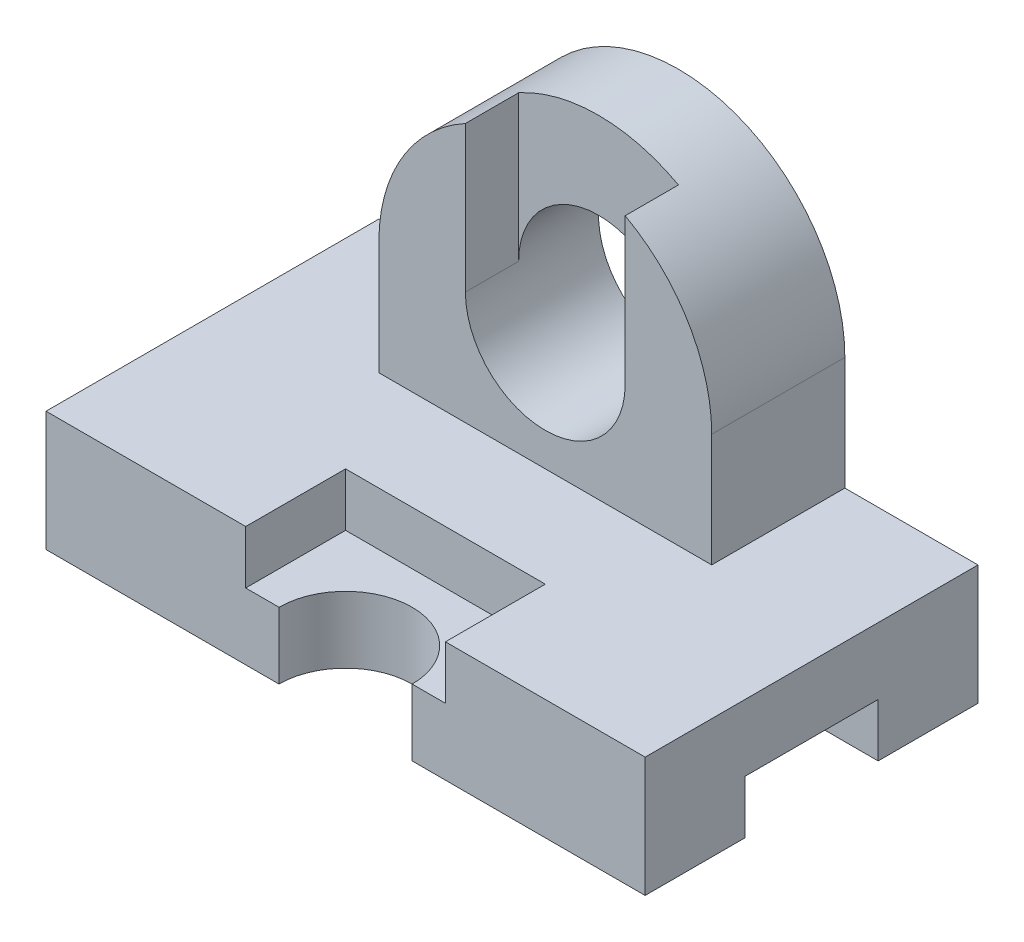
ISO-10303-21;
HEADER;
FILE_DESCRIPTION(('STEP AP214'),'2;1');
FILE_NAME('part.step','',(''),(''),'','','');
FILE_SCHEMA(('AUTOMOTIVE_DESIGN { 1 0 10303 214 1 1 1 1 }'));
ENDSEC;
DATA;
#1=APPLICATION_CONTEXT('core data for automotive mechanical design processes');
#2=APPLICATION_PROTOCOL_DEFINITION('international standard','automotive_design',2000,#1);
#3=PRODUCT_CONTEXT('',#1,'mechanical');
#4=PRODUCT('Part','Part','',(#3));
#5=PRODUCT_RELATED_PRODUCT_CATEGORY('part','',(#4));
#6=PRODUCT_DEFINITION_FORMATION('','',#4);
#7=PRODUCT_DEFINITION_CONTEXT('part definition',#1,'design');
#8=PRODUCT_DEFINITION('design','',#6,#7);
#9=PRODUCT_DEFINITION_SHAPE('','',#8);
#10=(LENGTH_UNIT() NAMED_UNIT(*) SI_UNIT(.MILLI.,.METRE.));
#11=(NAMED_UNIT(*) PLANE_ANGLE_UNIT() SI_UNIT($,.RADIAN.));
#12=(NAMED_UNIT(*) SI_UNIT($,.STERADIAN.) SOLID_ANGLE_UNIT());
#13=UNCERTAINTY_MEASURE_WITH_UNIT(LENGTH_MEASURE(1.E-05),#10,'distance_accuracy_value','');
#14=(GEOMETRIC_REPRESENTATION_CONTEXT(3) GLOBAL_UNCERTAINTY_ASSIGNED_CONTEXT((#13)) GLOBAL_UNIT_ASSIGNED_CONTEXT((#10,
#11,#12)) REPRESENTATION_CONTEXT('',''));
#15=CARTESIAN_POINT('',(0.,0.,0.));
#16=DIRECTION('',(0.,0.,1.));
#17=DIRECTION('',(1.,0.,0.));
#18=AXIS2_PLACEMENT_3D('',#15,#16,#17);
#19=CARTESIAN_POINT('',(0.,0.,50.));
#20=DIRECTION('',(0.,0.,1.));
#21=DIRECTION('',(1.,0.,0.));
#22=AXIS2_PLACEMENT_3D('',#19,#20,#21);
#23=PLANE('',#22);
#24=DIRECTION('',(0.,1.,0.));
#25=VECTOR('',#24,1.);
#26=CARTESIAN_POINT('',(55.,0.,50.));
#27=LINE('',#26,#25);
#28=CARTESIAN_POINT('',(55.,0.,50.));
#29=VERTEX_POINT('',#28);
#30=CARTESIAN_POINT('',(55.,10.,50.));
#31=VERTEX_POINT('',#30);
#32=EDGE_CURVE('E57',#29,#31,#27,.T.);
#33=ORIENTED_EDGE('',*,*,#32,.F.);
#34=DIRECTION('',(1.,0.,0.));
#35=VECTOR('',#34,1.);
#36=CARTESIAN_POINT('',(0.,0.,50.));
#37=LINE('',#36,#35);
#38=CARTESIAN_POINT('',(90.,0.,50.));
#39=VERTEX_POINT('',#38);
#40=EDGE_CURVE('E201',#29,#39,#37,.T.);
#41=ORIENTED_EDGE('',*,*,#40,.T.);
#42=DIRECTION('',(0.,1.,0.));
#43=VECTOR('',#42,1.);
#44=CARTESIAN_POINT('',(90.,0.,50.));
#45=LINE('',#44,#43);
#46=CARTESIAN_POINT('',(90.,18.,50.));
#47=VERTEX_POINT('',#46);
#48=EDGE_CURVE('E213',#39,#47,#45,.T.);
#49=ORIENTED_EDGE('',*,*,#48,.T.);
#50=DIRECTION('',(-1.,0.,0.));
#51=VECTOR('',#50,1.);
#52=CARTESIAN_POINT('',(90.,18.,50.));
#53=LINE('',#52,#51);
#54=CARTESIAN_POINT('',(60.,18.,50.));
#55=VERTEX_POINT('',#54);
#56=EDGE_CURVE('E223',#47,#55,#53,.T.);
#57=ORIENTED_EDGE('',*,*,#56,.T.);
#58=DIRECTION('',(0.,1.,0.));
#59=VECTOR('',#58,1.);
#60=CARTESIAN_POINT('',(60.,10.,50.));
#61=LINE('',#60,#59);
#62=CARTESIAN_POINT('',(60.,10.,50.));
#63=VERTEX_POINT('',#62);
#64=EDGE_CURVE('E273',#63,#55,#61,.T.);
#65=ORIENTED_EDGE('',*,*,#64,.F.);
#66=DIRECTION('',(1.,0.,0.));
#67=VECTOR('',#66,1.);
#68=CARTESIAN_POINT('',(30.,10.,50.));
#69=LINE('',#68,#67);
#70=EDGE_CURVE('E202',#31,#63,#69,.T.);
#71=ORIENTED_EDGE('',*,*,#70,.F.);
#72=EDGE_LOOP('',(#33,#41,#49,#57,#65,#71));
#73=FACE_BOUND('',#72,.T.);
#74=ADVANCED_FACE('F41',(#73),#23,.T.);
#75=CARTESIAN_POINT('',(0.,0.,50.));
#76=DIRECTION('',(0.,1.,0.));
#77=DIRECTION('',(0.,0.,1.));
#78=AXIS2_PLACEMENT_3D('',#75,#76,#77);
#79=PLANE('',#78);
#80=ORIENTED_EDGE('',*,*,#40,.F.);
#81=CARTESIAN_POINT('',(45.,0.,50.));
#82=DIRECTION('',(0.,1.,0.));
#83=DIRECTION('',(0.,0.,1.));
#84=AXIS2_PLACEMENT_3D('',#81,#82,#83);
#85=CIRCLE('',#84,10.);
#86=CARTESIAN_POINT('',(35.,0.,50.));
#87=VERTEX_POINT('',#86);
#88=EDGE_CURVE('E188',#29,#87,#85,.T.);
#89=ORIENTED_EDGE('',*,*,#88,.T.);
#90=CARTESIAN_POINT('',(0.,0.,50.));
#91=VERTEX_POINT('',#90);
#92=EDGE_CURVE('E215',#91,#87,#37,.T.);
#93=ORIENTED_EDGE('',*,*,#92,.F.);
#94=DIRECTION('',(0.,0.,-1.));
#95=VECTOR('',#94,1.);
#96=CARTESIAN_POINT('',(0.,0.,50.));
#97=LINE('',#96,#95);
#98=CARTESIAN_POINT('',(0.,0.,35.));
#99=VERTEX_POINT('',#98);
#100=EDGE_CURVE('E11',#91,#99,#97,.T.);
#101=ORIENTED_EDGE('',*,*,#100,.T.);
#102=DIRECTION('',(1.,0.,0.));
#103=VECTOR('',#102,1.);
#104=CARTESIAN_POINT('',(0.,0.,35.));
#105=LINE('',#104,#103);
#106=CARTESIAN_POINT('',(90.,0.,35.));
#107=VERTEX_POINT('',#106);
#108=EDGE_CURVE('E335',#99,#107,#105,.T.);
#109=ORIENTED_EDGE('',*,*,#108,.T.);
#110=DIRECTION('',(0.,0.,-1.));
#111=VECTOR('',#110,1.);
#112=CARTESIAN_POINT('',(90.,0.,50.));
#113=LINE('',#112,#111);
#114=EDGE_CURVE('E208',#39,#107,#113,.T.);
#115=ORIENTED_EDGE('',*,*,#114,.F.);
#116=EDGE_LOOP('',(#80,#89,#93,#101,#109,#115));
#117=FACE_BOUND('',#116,.T.);
#118=ADVANCED_FACE('F210',(#117),#79,.F.);
#119=CARTESIAN_POINT('',(90.,18.,50.));
#120=DIRECTION('',(0.,-1.,0.));
#121=DIRECTION('',(0.,0.,-1.));
#122=AXIS2_PLACEMENT_3D('',#119,#120,#121);
#123=PLANE('',#122);
#124=DIRECTION('',(-1.,0.,0.));
#125=VECTOR('',#124,1.);
#126=CARTESIAN_POINT('',(30.,18.,35.));
#127=LINE('',#126,#125);
#128=CARTESIAN_POINT('',(60.,18.,35.));
#129=VERTEX_POINT('',#128);
#130=CARTESIAN_POINT('',(30.,18.,35.));
#131=VERTEX_POINT('',#130);
#132=EDGE_CURVE('E386',#129,#131,#127,.T.);
#133=ORIENTED_EDGE('',*,*,#132,.F.);
#134=DIRECTION('',(0.,0.,-1.));
#135=VECTOR('',#134,1.);
#136=CARTESIAN_POINT('',(60.,18.,35.));
#137=LINE('',#136,#135);
#138=EDGE_CURVE('E204',#55,#129,#137,.T.);
#139=ORIENTED_EDGE('',*,*,#138,.F.);
#140=ORIENTED_EDGE('',*,*,#56,.F.);
#141=DIRECTION('',(0.,0.,-1.));
#142=VECTOR('',#141,1.);
#143=CARTESIAN_POINT('',(90.,18.,50.));
#144=LINE('',#143,#142);
#145=CARTESIAN_POINT('',(90.,18.,0.));
#146=VERTEX_POINT('',#145);
#147=EDGE_CURVE('E241',#47,#146,#144,.T.);
#148=ORIENTED_EDGE('',*,*,#147,.T.);
#149=DIRECTION('',(-1.,0.,0.));
#150=VECTOR('',#149,1.);
#151=CARTESIAN_POINT('',(90.,18.,0.));
#152=LINE('',#151,#150);
#153=CARTESIAN_POINT('',(70.,18.,0.));
#154=VERTEX_POINT('',#153);
#155=EDGE_CURVE('E220',#146,#154,#152,.T.);
#156=ORIENTED_EDGE('',*,*,#155,.T.);
#157=DIRECTION('',(0.,0.,-1.));
#158=VECTOR('',#157,1.);
#159=CARTESIAN_POINT('',(70.,18.,20.));
#160=LINE('',#159,#158);
#161=CARTESIAN_POINT('',(70.,18.,20.));
#162=VERTEX_POINT('',#161);
#163=EDGE_CURVE('E275',#162,#154,#160,.T.);
#164=ORIENTED_EDGE('',*,*,#163,.F.);
#165=DIRECTION('',(1.,0.,0.));
#166=VECTOR('',#165,1.);
#167=CARTESIAN_POINT('',(20.,18.,20.));
#168=LINE('',#167,#166);
#169=CARTESIAN_POINT('',(20.,18.,20.));
#170=VERTEX_POINT('',#169);
#171=EDGE_CURVE('E355',#170,#162,#168,.T.);
#172=ORIENTED_EDGE('',*,*,#171,.F.);
#173=DIRECTION('',(0.,0.,-1.));
#174=VECTOR('',#173,1.);
#175=CARTESIAN_POINT('',(20.,18.,20.));
#176=LINE('',#175,#174);
#177=CARTESIAN_POINT('',(20.,18.,0.));
#178=VERTEX_POINT('',#177);
#179=EDGE_CURVE('E362',#170,#178,#176,.T.);
#180=ORIENTED_EDGE('',*,*,#179,.T.);
#181=CARTESIAN_POINT('',(0.,18.,0.));
#182=VERTEX_POINT('',#181);
#183=EDGE_CURVE('E236',#178,#182,#152,.T.);
#184=ORIENTED_EDGE('',*,*,#183,.T.);
#185=DIRECTION('',(0.,0.,-1.));
#186=VECTOR('',#185,1.);
#187=CARTESIAN_POINT('',(0.,18.,50.));
#188=LINE('',#187,#186);
#189=CARTESIAN_POINT('',(0.,18.,50.));
#190=VERTEX_POINT('',#189);
#191=EDGE_CURVE('E228',#190,#182,#188,.T.);
#192=ORIENTED_EDGE('',*,*,#191,.F.);
#193=CARTESIAN_POINT('',(30.,18.,50.));
#194=VERTEX_POINT('',#193);
#195=EDGE_CURVE('E225',#194,#190,#53,.T.);
#196=ORIENTED_EDGE('',*,*,#195,.F.);
#197=DIRECTION('',(0.,0.,1.));
#198=VECTOR('',#197,1.);
#199=CARTESIAN_POINT('',(30.,18.,35.));
#200=LINE('',#199,#198);
#201=EDGE_CURVE('E288',#131,#194,#200,.T.);
#202=ORIENTED_EDGE('',*,*,#201,.F.);
#203=EDGE_LOOP('',(#133,#139,#140,#148,#156,#164,#172,#180,#184,#192,#196,#202));
#204=FACE_BOUND('',#203,.T.);
#205=ADVANCED_FACE('F269',(#204),#123,.F.);
#206=CARTESIAN_POINT('',(0.,18.,50.));
#207=DIRECTION('',(1.,0.,0.));
#208=DIRECTION('',(0.,0.,-1.));
#209=AXIS2_PLACEMENT_3D('',#206,#207,#208);
#210=PLANE('',#209);
#211=DIRECTION('',(0.,0.,1.));
#212=VECTOR('',#211,1.);
#213=CARTESIAN_POINT('',(0.,8.,35.));
#214=LINE('',#213,#212);
#215=CARTESIAN_POINT('',(0.,8.,15.));
#216=VERTEX_POINT('',#215);
#217=CARTESIAN_POINT('',(0.,8.,35.));
#218=VERTEX_POINT('',#217);
#219=EDGE_CURVE('E316',#216,#218,#214,.T.);
#220=ORIENTED_EDGE('',*,*,#219,.T.);
#221=DIRECTION('',(0.,-1.,0.));
#222=VECTOR('',#221,1.);
#223=CARTESIAN_POINT('',(0.,0.,35.));
#224=LINE('',#223,#222);
#225=EDGE_CURVE('E324',#218,#99,#224,.T.);
#226=ORIENTED_EDGE('',*,*,#225,.T.);
#227=ORIENTED_EDGE('',*,*,#100,.F.);
#228=DIRECTION('',(0.,-1.,0.));
#229=VECTOR('',#228,1.);
#230=CARTESIAN_POINT('',(0.,18.,50.));
#231=LINE('',#230,#229);
#232=EDGE_CURVE('E214',#190,#91,#231,.T.);
#233=ORIENTED_EDGE('',*,*,#232,.F.);
#234=ORIENTED_EDGE('',*,*,#191,.T.);
#235=DIRECTION('',(0.,-1.,0.));
#236=VECTOR('',#235,1.);
#237=CARTESIAN_POINT('',(0.,18.,0.));
#238=LINE('',#237,#236);
#239=CARTESIAN_POINT('',(0.,0.,0.));
#240=VERTEX_POINT('',#239);
#241=EDGE_CURVE('E227',#182,#240,#238,.T.);
#242=ORIENTED_EDGE('',*,*,#241,.T.);
#243=CARTESIAN_POINT('',(0.,0.,15.));
#244=VERTEX_POINT('',#243);
#245=EDGE_CURVE('E47',#244,#240,#97,.T.);
#246=ORIENTED_EDGE('',*,*,#245,.F.);
#247=DIRECTION('',(0.,1.,0.));
#248=VECTOR('',#247,1.);
#249=CARTESIAN_POINT('',(0.,8.,15.));
#250=LINE('',#249,#248);
#251=EDGE_CURVE('E317',#244,#216,#250,.T.);
#252=ORIENTED_EDGE('',*,*,#251,.T.);
#253=EDGE_LOOP('',(#220,#226,#227,#233,#234,#242,#246,#252));
#254=FACE_BOUND('',#253,.T.);
#255=ADVANCED_FACE('F43',(#254),#210,.F.);
#256=CARTESIAN_POINT('',(90.,0.,15.));
#257=VERTEX_POINT('',#256);
#258=CARTESIAN_POINT('',(90.,0.,0.));
#259=VERTEX_POINT('',#258);
#260=EDGE_CURVE('E243',#257,#259,#113,.T.);
#261=ORIENTED_EDGE('',*,*,#260,.F.);
#262=DIRECTION('',(1.,0.,0.));
#263=VECTOR('',#262,1.);
#264=CARTESIAN_POINT('',(0.,0.,15.));
#265=LINE('',#264,#263);
#266=EDGE_CURVE('E326',#244,#257,#265,.T.);
#267=ORIENTED_EDGE('',*,*,#266,.F.);
#268=ORIENTED_EDGE('',*,*,#245,.T.);
#269=DIRECTION('',(1.,0.,0.));
#270=VECTOR('',#269,1.);
#271=CARTESIAN_POINT('',(0.,0.,0.));
#272=LINE('',#271,#270);
#273=EDGE_CURVE('E229',#240,#259,#272,.T.);
#274=ORIENTED_EDGE('',*,*,#273,.T.);
#275=EDGE_LOOP('',(#261,#267,#268,#274));
#276=FACE_BOUND('',#275,.T.);
#277=ADVANCED_FACE('F260',(#276),#79,.F.);
#278=CARTESIAN_POINT('',(90.,0.,50.));
#279=DIRECTION('',(-1.,0.,0.));
#280=DIRECTION('',(0.,0.,1.));
#281=AXIS2_PLACEMENT_3D('',#278,#279,#280);
#282=PLANE('',#281);
#283=ORIENTED_EDGE('',*,*,#114,.T.);
#284=DIRECTION('',(0.,-1.,0.));
#285=VECTOR('',#284,1.);
#286=CARTESIAN_POINT('',(90.,0.,35.));
#287=LINE('',#286,#285);
#288=CARTESIAN_POINT('',(90.,8.,35.));
#289=VERTEX_POINT('',#288);
#290=EDGE_CURVE('E318',#289,#107,#287,.T.);
#291=ORIENTED_EDGE('',*,*,#290,.F.);
#292=DIRECTION('',(0.,0.,1.));
#293=VECTOR('',#292,1.);
#294=CARTESIAN_POINT('',(90.,8.,35.));
#295=LINE('',#294,#293);
#296=CARTESIAN_POINT('',(90.,8.,15.));
#297=VERTEX_POINT('',#296);
#298=EDGE_CURVE('E328',#297,#289,#295,.T.);
#299=ORIENTED_EDGE('',*,*,#298,.F.);
#300=DIRECTION('',(0.,1.,0.));
#301=VECTOR('',#300,1.);
#302=CARTESIAN_POINT('',(90.,8.,15.));
#303=LINE('',#302,#301);
#304=EDGE_CURVE('E254',#257,#297,#303,.T.);
#305=ORIENTED_EDGE('',*,*,#304,.F.);
#306=ORIENTED_EDGE('',*,*,#260,.T.);
#307=DIRECTION('',(0.,1.,0.));
#308=VECTOR('',#307,1.);
#309=CARTESIAN_POINT('',(90.,0.,0.));
#310=LINE('',#309,#308);
#311=EDGE_CURVE('E234',#259,#146,#310,.T.);
#312=ORIENTED_EDGE('',*,*,#311,.T.);
#313=ORIENTED_EDGE('',*,*,#147,.F.);
#314=ORIENTED_EDGE('',*,*,#48,.F.);
#315=EDGE_LOOP('',(#283,#291,#299,#305,#306,#312,#313,#314));
#316=FACE_BOUND('',#315,.T.);
#317=ADVANCED_FACE('F247',(#316),#282,.F.);
#318=DIRECTION('',(0.,1.,0.));
#319=VECTOR('',#318,1.);
#320=CARTESIAN_POINT('',(35.,0.,50.));
#321=LINE('',#320,#319);
#322=CARTESIAN_POINT('',(35.,10.,50.));
#323=VERTEX_POINT('',#322);
#324=EDGE_CURVE('E194',#323,#87,#321,.F.);
#325=ORIENTED_EDGE('',*,*,#324,.F.);
#326=CARTESIAN_POINT('',(30.,10.,50.));
#327=VERTEX_POINT('',#326);
#328=EDGE_CURVE('E295',#327,#323,#69,.T.);
#329=ORIENTED_EDGE('',*,*,#328,.F.);
#330=DIRECTION('',(0.,1.,0.));
#331=VECTOR('',#330,1.);
#332=CARTESIAN_POINT('',(30.,10.,50.));
#333=LINE('',#332,#331);
#334=EDGE_CURVE('E278',#327,#194,#333,.T.);
#335=ORIENTED_EDGE('',*,*,#334,.T.);
#336=ORIENTED_EDGE('',*,*,#195,.T.);
#337=ORIENTED_EDGE('',*,*,#232,.T.);
#338=ORIENTED_EDGE('',*,*,#92,.T.);
#339=EDGE_LOOP('',(#325,#329,#335,#336,#337,#338));
#340=FACE_BOUND('',#339,.T.);
#341=ADVANCED_FACE('F383',(#340),#23,.T.);
#342=CARTESIAN_POINT('',(0.,0.,0.));
#343=DIRECTION('',(0.,0.,1.));
#344=DIRECTION('',(1.,0.,0.));
#345=AXIS2_PLACEMENT_3D('',#342,#343,#344);
#346=PLANE('',#345);
#347=ORIENTED_EDGE('',*,*,#241,.F.);
#348=ORIENTED_EDGE('',*,*,#183,.F.);
#349=DIRECTION('',(0.,-1.,0.));
#350=VECTOR('',#349,1.);
#351=CARTESIAN_POINT('',(20.,35.,0.));
#352=LINE('',#351,#350);
#353=CARTESIAN_POINT('',(20.,35.,0.));
#354=VERTEX_POINT('',#353);
#355=EDGE_CURVE('E360',#354,#178,#352,.T.);
#356=ORIENTED_EDGE('',*,*,#355,.F.);
#357=CARTESIAN_POINT('',(45.,35.,0.));
#358=DIRECTION('',(0.,0.,1.));
#359=DIRECTION('',(1.,0.,0.));
#360=AXIS2_PLACEMENT_3D('',#357,#358,#359);
#361=CIRCLE('',#360,25.);
#362=CARTESIAN_POINT('',(70.,35.,0.));
#363=VERTEX_POINT('',#362);
#364=EDGE_CURVE('E344',#363,#354,#361,.T.);
#365=ORIENTED_EDGE('',*,*,#364,.F.);
#366=DIRECTION('',(0.,1.,0.));
#367=VECTOR('',#366,1.);
#368=CARTESIAN_POINT('',(70.,35.,0.));
#369=LINE('',#368,#367);
#370=EDGE_CURVE('E266',#154,#363,#369,.T.);
#371=ORIENTED_EDGE('',*,*,#370,.F.);
#372=ORIENTED_EDGE('',*,*,#155,.F.);
#373=ORIENTED_EDGE('',*,*,#311,.F.);
#374=ORIENTED_EDGE('',*,*,#273,.F.);
#375=EDGE_LOOP('',(#347,#348,#356,#365,#371,#372,#373,#374));
#376=FACE_BOUND('',#375,.T.);
#377=CARTESIAN_POINT('',(45.,35.,0.));
#378=DIRECTION('',(0.,0.,1.));
#379=DIRECTION('',(1.,0.,0.));
#380=AXIS2_PLACEMENT_3D('',#377,#378,#379);
#381=CIRCLE('',#380,12.);
#382=CARTESIAN_POINT('',(57.,35.,0.));
#383=VERTEX_POINT('',#382);
#384=EDGE_CURVE('E332',#383,#383,#381,.T.);
#385=ORIENTED_EDGE('',*,*,#384,.T.);
#386=EDGE_LOOP('',(#385));
#387=FACE_BOUND('',#386,.T.);
#388=ADVANCED_FACE('F265',(#376,#387),#346,.F.);
#389=CARTESIAN_POINT('',(45.,35.,20.));
#390=DIRECTION('',(0.,0.,1.));
#391=DIRECTION('',(1.,0.,0.));
#392=AXIS2_PLACEMENT_3D('',#389,#390,#391);
#393=PLANE('',#392);
#394=DIRECTION('',(0.,-1.,0.));
#395=VECTOR('',#394,1.);
#396=CARTESIAN_POINT('',(33.,35.,20.));
#397=LINE('',#396,#395);
#398=CARTESIAN_POINT('',(33.,56.9317121994613,20.));
#399=VERTEX_POINT('',#398);
#400=CARTESIAN_POINT('',(33.,35.,20.));
#401=VERTEX_POINT('',#400);
#402=EDGE_CURVE('E285',#399,#401,#397,.T.);
#403=ORIENTED_EDGE('',*,*,#402,.F.);
#404=CARTESIAN_POINT('',(45.,35.,20.));
#405=DIRECTION('',(0.,0.,1.));
#406=DIRECTION('',(1.,0.,0.));
#407=AXIS2_PLACEMENT_3D('',#404,#405,#406);
#408=CIRCLE('',#407,25.);
#409=CARTESIAN_POINT('',(20.,35.,20.));
#410=VERTEX_POINT('',#409);
#411=EDGE_CURVE('E349',#399,#410,#408,.T.);
#412=ORIENTED_EDGE('',*,*,#411,.T.);
#413=DIRECTION('',(0.,-1.,0.));
#414=VECTOR('',#413,1.);
#415=CARTESIAN_POINT('',(20.,35.,20.));
#416=LINE('',#415,#414);
#417=EDGE_CURVE('E347',#410,#170,#416,.T.);
#418=ORIENTED_EDGE('',*,*,#417,.T.);
#419=ORIENTED_EDGE('',*,*,#171,.T.);
#420=DIRECTION('',(0.,1.,0.));
#421=VECTOR('',#420,1.);
#422=CARTESIAN_POINT('',(70.,35.,20.));
#423=LINE('',#422,#421);
#424=CARTESIAN_POINT('',(70.,35.,20.));
#425=VERTEX_POINT('',#424);
#426=EDGE_CURVE('E352',#162,#425,#423,.T.);
#427=ORIENTED_EDGE('',*,*,#426,.T.);
#428=CARTESIAN_POINT('',(57.,56.9317121994613,20.));
#429=VERTEX_POINT('',#428);
#430=EDGE_CURVE('E346',#425,#429,#408,.T.);
#431=ORIENTED_EDGE('',*,*,#430,.T.);
#432=DIRECTION('',(0.,1.,0.));
#433=VECTOR('',#432,1.);
#434=CARTESIAN_POINT('',(57.,35.,20.));
#435=LINE('',#434,#433);
#436=CARTESIAN_POINT('',(57.,35.,20.));
#437=VERTEX_POINT('',#436);
#438=EDGE_CURVE('E276',#437,#429,#435,.T.);
#439=ORIENTED_EDGE('',*,*,#438,.F.);
#440=CARTESIAN_POINT('',(45.,35.,20.));
#441=DIRECTION('',(0.,0.,1.));
#442=DIRECTION('',(1.,0.,0.));
#443=AXIS2_PLACEMENT_3D('',#440,#441,#442);
#444=CIRCLE('',#443,12.);
#445=EDGE_CURVE('E338',#401,#437,#444,.T.);
#446=ORIENTED_EDGE('',*,*,#445,.F.);
#447=EDGE_LOOP('',(#403,#412,#418,#419,#427,#431,#439,#446));
#448=FACE_BOUND('',#447,.T.);
#449=ADVANCED_FACE('F424',(#448),#393,.T.);
#450=CARTESIAN_POINT('',(45.,35.,20.));
#451=DIRECTION('',(0.,0.,-1.));
#452=DIRECTION('',(-1.,0.,0.));
#453=AXIS2_PLACEMENT_3D('',#450,#451,#452);
#454=CYLINDRICAL_SURFACE('',#453,25.);
#455=ORIENTED_EDGE('',*,*,#411,.F.);
#456=DIRECTION('',(0.,0.,1.));
#457=VECTOR('',#456,1.);
#458=CARTESIAN_POINT('',(33.,56.9317121994613,12.));
#459=LINE('',#458,#457);
#460=CARTESIAN_POINT('',(33.,56.9317121994613,12.));
#461=VERTEX_POINT('',#460);
#462=EDGE_CURVE('E309',#461,#399,#459,.T.);
#463=ORIENTED_EDGE('',*,*,#462,.F.);
#464=CARTESIAN_POINT('',(45.,34.9999999999993,12.));
#465=DIRECTION('',(0.,0.,1.));
#466=DIRECTION('',(-1.,0.,0.));
#467=AXIS2_PLACEMENT_3D('',#464,#465,#466);
#468=CIRCLE('',#467,25.0000000000006);
#469=CARTESIAN_POINT('',(57.,56.9317121994613,12.));
#470=VERTEX_POINT('',#469);
#471=EDGE_CURVE('E301',#470,#461,#468,.T.);
#472=ORIENTED_EDGE('',*,*,#471,.F.);
#473=DIRECTION('',(0.,0.,1.));
#474=VECTOR('',#473,1.);
#475=CARTESIAN_POINT('',(57.,56.9317121994613,12.));
#476=LINE('',#475,#474);
#477=EDGE_CURVE('E315',#470,#429,#476,.T.);
#478=ORIENTED_EDGE('',*,*,#477,.T.);
#479=ORIENTED_EDGE('',*,*,#430,.F.);
#480=DIRECTION('',(0.,0.,-1.));
#481=VECTOR('',#480,1.);
#482=CARTESIAN_POINT('',(70.,35.,20.));
#483=LINE('',#482,#481);
#484=EDGE_CURVE('E358',#425,#363,#483,.T.);
#485=ORIENTED_EDGE('',*,*,#484,.T.);
#486=ORIENTED_EDGE('',*,*,#364,.T.);
#487=DIRECTION('',(0.,0.,-1.));
#488=VECTOR('',#487,1.);
#489=CARTESIAN_POINT('',(20.,35.,20.));
#490=LINE('',#489,#488);
#491=EDGE_CURVE('E233',#410,#354,#490,.T.);
#492=ORIENTED_EDGE('',*,*,#491,.F.);
#493=EDGE_LOOP('',(#455,#463,#472,#478,#479,#485,#486,#492));
#494=FACE_BOUND('',#493,.T.);
#495=ADVANCED_FACE('F374',(#494),#454,.T.);
#496=CARTESIAN_POINT('',(20.,35.,20.));
#497=DIRECTION('',(1.,0.,0.));
#498=DIRECTION('',(0.,1.,0.));
#499=AXIS2_PLACEMENT_3D('',#496,#497,#498);
#500=PLANE('',#499);
#501=ORIENTED_EDGE('',*,*,#355,.T.);
#502=ORIENTED_EDGE('',*,*,#179,.F.);
#503=ORIENTED_EDGE('',*,*,#417,.F.);
#504=ORIENTED_EDGE('',*,*,#491,.T.);
#505=EDGE_LOOP('',(#501,#502,#503,#504));
#506=FACE_BOUND('',#505,.T.);
#507=ADVANCED_FACE('F371',(#506),#500,.F.);
#508=CARTESIAN_POINT('',(70.,35.,20.));
#509=DIRECTION('',(-1.,0.,0.));
#510=DIRECTION('',(0.,-1.,0.));
#511=AXIS2_PLACEMENT_3D('',#508,#509,#510);
#512=PLANE('',#511);
#513=ORIENTED_EDGE('',*,*,#370,.T.);
#514=ORIENTED_EDGE('',*,*,#484,.F.);
#515=ORIENTED_EDGE('',*,*,#426,.F.);
#516=ORIENTED_EDGE('',*,*,#163,.T.);
#517=EDGE_LOOP('',(#513,#514,#515,#516));
#518=FACE_BOUND('',#517,.T.);
#519=ADVANCED_FACE('F447',(#518),#512,.F.);
#520=CARTESIAN_POINT('',(45.,35.,20.));
#521=DIRECTION('',(0.,0.,-1.));
#522=DIRECTION('',(-1.,0.,0.));
#523=AXIS2_PLACEMENT_3D('',#520,#521,#522);
#524=CYLINDRICAL_SURFACE('',#523,12.);
#525=DIRECTION('',(0.,0.,1.));
#526=VECTOR('',#525,1.);
#527=CARTESIAN_POINT('',(33.,35.,12.));
#528=LINE('',#527,#526);
#529=CARTESIAN_POINT('',(33.,35.,12.));
#530=VERTEX_POINT('',#529);
#531=EDGE_CURVE('E310',#530,#401,#528,.T.);
#532=ORIENTED_EDGE('',*,*,#531,.T.);
#533=ORIENTED_EDGE('',*,*,#445,.T.);
#534=DIRECTION('',(0.,0.,1.));
#535=VECTOR('',#534,1.);
#536=CARTESIAN_POINT('',(57.,35.,12.));
#537=LINE('',#536,#535);
#538=CARTESIAN_POINT('',(57.,35.,12.));
#539=VERTEX_POINT('',#538);
#540=EDGE_CURVE('E302',#539,#437,#537,.T.);
#541=ORIENTED_EDGE('',*,*,#540,.F.);
#542=CARTESIAN_POINT('',(45.,35.,12.));
#543=DIRECTION('',(0.,0.,-1.));
#544=DIRECTION('',(-1.,0.,0.));
#545=AXIS2_PLACEMENT_3D('',#542,#543,#544);
#546=CIRCLE('',#545,12.);
#547=EDGE_CURVE('E294',#530,#539,#546,.T.);
#548=ORIENTED_EDGE('',*,*,#547,.F.);
#549=EDGE_LOOP('',(#532,#533,#541,#548));
#550=FACE_BOUND('',#549,.T.);
#551=ORIENTED_EDGE('',*,*,#384,.F.);
#552=EDGE_LOOP('',(#551));
#553=FACE_BOUND('',#552,.T.);
#554=ADVANCED_FACE('F498',(#550,#553),#524,.F.);
#555=CARTESIAN_POINT('',(0.,0.,35.));
#556=DIRECTION('',(0.,0.,1.));
#557=DIRECTION('',(1.,0.,0.));
#558=AXIS2_PLACEMENT_3D('',#555,#556,#557);
#559=PLANE('',#558);
#560=ORIENTED_EDGE('',*,*,#290,.T.);
#561=ORIENTED_EDGE('',*,*,#108,.F.);
#562=ORIENTED_EDGE('',*,*,#225,.F.);
#563=DIRECTION('',(1.,0.,0.));
#564=VECTOR('',#563,1.);
#565=CARTESIAN_POINT('',(0.,8.,35.));
#566=LINE('',#565,#564);
#567=EDGE_CURVE('E334',#218,#289,#566,.T.);
#568=ORIENTED_EDGE('',*,*,#567,.T.);
#569=EDGE_LOOP('',(#560,#561,#562,#568));
#570=FACE_BOUND('',#569,.T.);
#571=ADVANCED_FACE('F510',(#570),#559,.F.);
#572=CARTESIAN_POINT('',(0.,8.,35.));
#573=DIRECTION('',(0.,1.,0.));
#574=DIRECTION('',(0.,0.,1.));
#575=AXIS2_PLACEMENT_3D('',#572,#573,#574);
#576=PLANE('',#575);
#577=ORIENTED_EDGE('',*,*,#298,.T.);
#578=ORIENTED_EDGE('',*,*,#567,.F.);
#579=ORIENTED_EDGE('',*,*,#219,.F.);
#580=DIRECTION('',(1.,0.,0.));
#581=VECTOR('',#580,1.);
#582=CARTESIAN_POINT('',(0.,8.,15.));
#583=LINE('',#582,#581);
#584=EDGE_CURVE('E340',#216,#297,#583,.T.);
#585=ORIENTED_EDGE('',*,*,#584,.T.);
#586=EDGE_LOOP('',(#577,#578,#579,#585));
#587=FACE_BOUND('',#586,.T.);
#588=ADVANCED_FACE('F521',(#587),#576,.F.);
#589=CARTESIAN_POINT('',(0.,8.,15.));
#590=DIRECTION('',(0.,0.,-1.));
#591=DIRECTION('',(0.,1.,0.));
#592=AXIS2_PLACEMENT_3D('',#589,#590,#591);
#593=PLANE('',#592);
#594=ORIENTED_EDGE('',*,*,#304,.T.);
#595=ORIENTED_EDGE('',*,*,#584,.F.);
#596=ORIENTED_EDGE('',*,*,#251,.F.);
#597=ORIENTED_EDGE('',*,*,#266,.T.);
#598=EDGE_LOOP('',(#594,#595,#596,#597));
#599=FACE_BOUND('',#598,.T.);
#600=ADVANCED_FACE('F529',(#599),#593,.F.);
#601=CARTESIAN_POINT('',(33.,35.,12.));
#602=DIRECTION('',(-1.,0.,0.));
#603=DIRECTION('',(0.,0.,1.));
#604=AXIS2_PLACEMENT_3D('',#601,#602,#603);
#605=PLANE('',#604);
#606=ORIENTED_EDGE('',*,*,#402,.T.);
#607=ORIENTED_EDGE('',*,*,#531,.F.);
#608=DIRECTION('',(0.,-1.,0.));
#609=VECTOR('',#608,1.);
#610=CARTESIAN_POINT('',(33.,35.,12.));
#611=LINE('',#610,#609);
#612=EDGE_CURVE('E303',#461,#530,#611,.T.);
#613=ORIENTED_EDGE('',*,*,#612,.F.);
#614=ORIENTED_EDGE('',*,*,#462,.T.);
#615=EDGE_LOOP('',(#606,#607,#613,#614));
#616=FACE_BOUND('',#615,.T.);
#617=ADVANCED_FACE('F536',(#616),#605,.F.);
#618=CARTESIAN_POINT('',(57.,35.,12.));
#619=DIRECTION('',(1.,0.,0.));
#620=DIRECTION('',(0.,0.,-1.));
#621=AXIS2_PLACEMENT_3D('',#618,#619,#620);
#622=PLANE('',#621);
#623=ORIENTED_EDGE('',*,*,#438,.T.);
#624=ORIENTED_EDGE('',*,*,#477,.F.);
#625=DIRECTION('',(0.,1.,0.));
#626=VECTOR('',#625,1.);
#627=CARTESIAN_POINT('',(57.,35.,12.));
#628=LINE('',#627,#626);
#629=EDGE_CURVE('E296',#539,#470,#628,.T.);
#630=ORIENTED_EDGE('',*,*,#629,.F.);
#631=ORIENTED_EDGE('',*,*,#540,.T.);
#632=EDGE_LOOP('',(#623,#624,#630,#631));
#633=FACE_BOUND('',#632,.T.);
#634=ADVANCED_FACE('F548',(#633),#622,.F.);
#635=CARTESIAN_POINT('',(45.,35.,12.));
#636=DIRECTION('',(0.,0.,-1.));
#637=DIRECTION('',(-1.,0.,0.));
#638=AXIS2_PLACEMENT_3D('',#635,#636,#637);
#639=PLANE('',#638);
#640=ORIENTED_EDGE('',*,*,#547,.T.);
#641=ORIENTED_EDGE('',*,*,#629,.T.);
#642=ORIENTED_EDGE('',*,*,#471,.T.);
#643=ORIENTED_EDGE('',*,*,#612,.T.);
#644=EDGE_LOOP('',(#640,#641,#642,#643));
#645=FACE_BOUND('',#644,.T.);
#646=ADVANCED_FACE('F560',(#645),#639,.F.);
#647=CARTESIAN_POINT('',(60.,10.,35.));
#648=DIRECTION('',(1.,0.,0.));
#649=DIRECTION('',(0.,0.,-1.));
#650=AXIS2_PLACEMENT_3D('',#647,#648,#649);
#651=PLANE('',#650);
#652=ORIENTED_EDGE('',*,*,#138,.T.);
#653=DIRECTION('',(0.,1.,0.));
#654=VECTOR('',#653,1.);
#655=CARTESIAN_POINT('',(60.,10.,35.));
#656=LINE('',#655,#654);
#657=CARTESIAN_POINT('',(60.,10.,35.));
#658=VERTEX_POINT('',#657);
#659=EDGE_CURVE('E292',#658,#129,#656,.T.);
#660=ORIENTED_EDGE('',*,*,#659,.F.);
#661=DIRECTION('',(0.,0.,-1.));
#662=VECTOR('',#661,1.);
#663=CARTESIAN_POINT('',(60.,10.,35.));
#664=LINE('',#663,#662);
#665=EDGE_CURVE('E391',#63,#658,#664,.T.);
#666=ORIENTED_EDGE('',*,*,#665,.F.);
#667=ORIENTED_EDGE('',*,*,#64,.T.);
#668=EDGE_LOOP('',(#652,#660,#666,#667));
#669=FACE_BOUND('',#668,.T.);
#670=ADVANCED_FACE('F564',(#669),#651,.F.);
#671=CARTESIAN_POINT('',(30.,10.,35.));
#672=DIRECTION('',(-1.,0.,0.));
#673=DIRECTION('',(0.,0.,1.));
#674=AXIS2_PLACEMENT_3D('',#671,#672,#673);
#675=PLANE('',#674);
#676=ORIENTED_EDGE('',*,*,#201,.T.);
#677=ORIENTED_EDGE('',*,*,#334,.F.);
#678=DIRECTION('',(0.,0.,1.));
#679=VECTOR('',#678,1.);
#680=CARTESIAN_POINT('',(30.,10.,35.));
#681=LINE('',#680,#679);
#682=CARTESIAN_POINT('',(30.,10.,35.));
#683=VERTEX_POINT('',#682);
#684=EDGE_CURVE('E61',#683,#327,#681,.T.);
#685=ORIENTED_EDGE('',*,*,#684,.F.);
#686=DIRECTION('',(0.,1.,0.));
#687=VECTOR('',#686,1.);
#688=CARTESIAN_POINT('',(30.,10.,35.));
#689=LINE('',#688,#687);
#690=EDGE_CURVE('E284',#683,#131,#689,.T.);
#691=ORIENTED_EDGE('',*,*,#690,.T.);
#692=EDGE_LOOP('',(#676,#677,#685,#691));
#693=FACE_BOUND('',#692,.T.);
#694=ADVANCED_FACE('F415',(#693),#675,.F.);
#695=CARTESIAN_POINT('',(30.,10.,35.));
#696=DIRECTION('',(0.,0.,-1.));
#697=DIRECTION('',(-1.,0.,0.));
#698=AXIS2_PLACEMENT_3D('',#695,#696,#697);
#699=PLANE('',#698);
#700=ORIENTED_EDGE('',*,*,#132,.T.);
#701=ORIENTED_EDGE('',*,*,#690,.F.);
#702=DIRECTION('',(-1.,0.,0.));
#703=VECTOR('',#702,1.);
#704=CARTESIAN_POINT('',(30.,10.,35.));
#705=LINE('',#704,#703);
#706=EDGE_CURVE('E393',#658,#683,#705,.T.);
#707=ORIENTED_EDGE('',*,*,#706,.F.);
#708=ORIENTED_EDGE('',*,*,#659,.T.);
#709=EDGE_LOOP('',(#700,#701,#707,#708));
#710=FACE_BOUND('',#709,.T.);
#711=ADVANCED_FACE('F404',(#710),#699,.F.);
#712=CARTESIAN_POINT('',(0.,10.,0.));
#713=DIRECTION('',(0.,1.,0.));
#714=DIRECTION('',(0.,0.,1.));
#715=AXIS2_PLACEMENT_3D('',#712,#713,#714);
#716=PLANE('',#715);
#717=CARTESIAN_POINT('',(45.,10.,50.));
#718=DIRECTION('',(0.,1.,0.));
#719=DIRECTION('',(0.,0.,1.));
#720=AXIS2_PLACEMENT_3D('',#717,#718,#719);
#721=CIRCLE('',#720,10.);
#722=EDGE_CURVE('E200',#31,#323,#721,.T.);
#723=ORIENTED_EDGE('',*,*,#722,.F.);
#724=ORIENTED_EDGE('',*,*,#70,.T.);
#725=ORIENTED_EDGE('',*,*,#665,.T.);
#726=ORIENTED_EDGE('',*,*,#706,.T.);
#727=ORIENTED_EDGE('',*,*,#684,.T.);
#728=ORIENTED_EDGE('',*,*,#328,.T.);
#729=EDGE_LOOP('',(#723,#724,#725,#726,#727,#728));
#730=FACE_BOUND('',#729,.T.);
#731=ADVANCED_FACE('F405',(#730),#716,.T.);
#732=CARTESIAN_POINT('',(45.,0.,50.));
#733=DIRECTION('',(0.,1.,0.));
#734=DIRECTION('',(0.,0.,1.));
#735=AXIS2_PLACEMENT_3D('',#732,#733,#734);
#736=CYLINDRICAL_SURFACE('',#735,10.);
#737=ORIENTED_EDGE('',*,*,#32,.T.);
#738=ORIENTED_EDGE('',*,*,#722,.T.);
#739=ORIENTED_EDGE('',*,*,#324,.T.);
#740=ORIENTED_EDGE('',*,*,#88,.F.);
#741=EDGE_LOOP('',(#737,#738,#739,#740));
#742=FACE_BOUND('',#741,.T.);
#743=ADVANCED_FACE('F192',(#742),#736,.F.);
#744=CLOSED_SHELL('',(#74,#118,#205,#255,#277,#317,#341,#388,#449,#495,#507,#519,#554,#571,#588,
#600,#617,#634,#646,#670,#694,#711,#731,#743));
#745=MANIFOLD_SOLID_BREP('B2',#744);
#746=ADVANCED_BREP_SHAPE_REPRESENTATION('',(#18,#745),#14);
#747=SHAPE_DEFINITION_REPRESENTATION(#9,#746);
ENDSEC;
END-ISO-10303-21;
